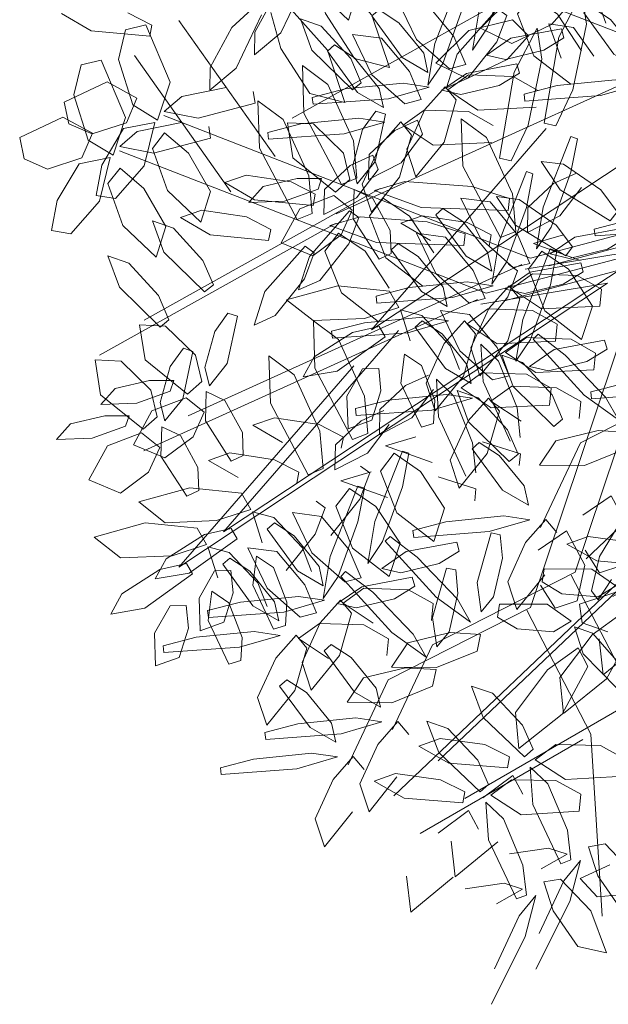
# Model space of a CAD drawing. Units: inches. Extents: x -48 to 50072, y 0 to 21068.
# Tile 72 of 75: x 2857 to 5091, y 14380 to 18117. Entities that reach past the tile are written whole.
import ezdxf

# ---------------------------------------------------------------- set-up
doc = ezdxf.new("R2010")
doc.units = ezdxf.units.IN
doc.header["$MEASUREMENT"] = 0
doc.layers.add('L-PLNT', color=94, linetype='Continuous', lineweight=13)

# ---------------------------------------------------------------- blocks, each defined once
blk = doc.blocks.new('A$C173E365C')
for p, q in [((1.5761, 3.6983), (1.6808, 3.966)), ((0.5021, 3.767), (0.4099, 3.8142)), ((0.8813, 3.8284), (0.8053, 3.758)), ((0.9917, 3.6783), (0.9528, 3.8156)), ((1.0318, 3.8259), (1.1681, 3.6723)), ((1.6811, 3.8304), (1.6056, 3.6222)), ((0.1587, 3.8117), (0.2714, 3.7462)), ((0.8218, 3.6045), (0.9181, 3.8063)), ((1.8711, 3.7875), (1.7053, 3.7467)), ((1.9311, 3.7273), (1.8711, 3.7875)), ((0.2714, 3.7462), (0.494, 3.7249)), ((0.494, 3.7249), (0.5021, 3.767)), ((0.8053, 3.758), (0.7232, 3.6071)), ((1.7053, 3.7467), (1.5796, 3.6226)), ((1.9642, 3.756), (1.8772, 3.589)), ((1.9823, 3.6377), (1.9642, 3.756)), ((2.0085, 3.7729), (2.1025, 3.7585)), ((2.0553, 3.6421), (2.0085, 3.7729)), ((2.1025, 3.7585), (2.18, 3.6496)), ((1.2636, 3.7321), (1.3739, 3.7178)), ((1.3371, 3.579), (1.2636, 3.7321)), ((1.3739, 3.7178), (1.4793, 3.5913)), ((1.8499, 3.6368), (1.9311, 3.7273)), ((1.1017, 3.5078), (0.9917, 3.6783)), ((1.168, 3.669), (1.1949, 3.6927)), ((1.2827, 3.5117), (1.168, 3.669)), ((1.1681, 3.6723), (1.2347, 3.4738)), ((1.1949, 3.6927), (1.2703, 3.6435)), ((1.5498, 3.5395), (1.5761, 3.6983)), ((0.3098, 3.635), (0.2331, 3.6169)), ((0.4015, 3.4171), (0.3098, 3.635)), ((0.8011, 3.1351), (0.4353, 3.6521)), ((1.2703, 3.6435), (1.3645, 3.5273)), ((1.6992, 3.5646), (1.8499, 3.6368)), ((1.93, 3.3883), (1.9823, 3.6377)), ((0.2331, 3.6169), (0.2056, 3.5033)), ((0.7232, 3.6071), (0.7217, 3.5211)), ((0.7217, 3.5211), (0.8218, 3.6045)), ((1.4793, 3.5913), (1.5243, 3.4847)), ((1.6056, 3.6222), (1.5498, 3.5395)), ((1.5796, 3.6226), (1.6992, 3.5646)), ((1.6957, 3.5841), (1.8871, 3.62)), ((1.8772, 3.589), (1.8217, 3.2626)), ((1.8871, 3.62), (1.8969, 3.5855)), ((1.4619, 3.4687), (1.3371, 3.579)), ((1.6023, 3.5204), (1.6957, 3.5841)), ((1.8969, 3.5855), (1.8201, 3.5387)), ((1.3645, 3.5273), (1.3805, 3.4548)), ((1.6746, 3.5036), (1.6023, 3.5204)), ((1.8201, 3.5387), (1.6746, 3.5036)), ((0.2056, 3.5033), (0.2599, 3.3313)), ((0.9042, 3.4803), (0.91, 3.3006)), ((1.0001, 3.4088), (0.9042, 3.4803)), ((1.2347, 3.4738), (1.1017, 3.5078)), ((1.3805, 3.4548), (1.2827, 3.5117)), ((1.5243, 3.4847), (1.4619, 3.4687)), ((1.535, 3.4449), (1.4557, 3.388)), ((1.704, 3.4392), (1.535, 3.4449)), ((1.7972, 3.3865), (1.704, 3.4392)), ((0.1633, 3.4186), (0, 3.3413)), ((0.2759, 3.3573), (0.1633, 3.4186)), ((0.3545, 3.2734), (0.4015, 3.4171)), ((1.0981, 3.1948), (1.0001, 3.4088)), ((1.0667, 3.3925), (1.2871, 3.414)), ((1.2871, 3.414), (1.3858, 3.3992)), ((0.6146, 3.3975), (0.4463, 3.3632)), ((0.7247, 3.338), (0.7176, 3.3828)), ((0.9414, 3.36), (1.0667, 3.3925)), ((1.3858, 3.3992), (1.2311, 3.3546)), ((1.3693, 3.3133), (1.4462, 3.3998)), ((1.4462, 3.3998), (1.4875, 3.3503)), ((1.4557, 3.388), (1.5699, 3.312)), ((1.8657, 3.2519), (1.93, 3.3883)), ((0, 3.3413), (0.0175, 3.2595)), ((0.2358, 3.2632), (0.2759, 3.3573)), ((0.2599, 3.3313), (0.3545, 3.2734)), ((0.4463, 3.3632), (0.3797, 3.3068)), ((0.5083, 3.2812), (0.7247, 3.338)), ((0.9444, 3.334), (0.9414, 3.36)), ((1.2311, 3.3546), (0.9444, 3.334)), ((1.4875, 3.3503), (1.4417, 3.1902)), ((1.7703, 2.7497), (0.3786, 3.2908)), ((0.3797, 3.3068), (0.5083, 3.2812)), ((0.91, 3.3006), (1.0531, 3.0294)), ((1.3005, 3.1637), (1.3693, 3.3133)), ((1.5699, 3.312), (1.7909, 3.3223)), ((0.0175, 3.2595), (0.1061, 3.221)), ((0.1061, 3.221), (0.2358, 3.2632)), ((0.3439, 3.2644), (0.2256, 3.2413)), ((0.3033, 3.0996), (0.3439, 3.2644)), ((1.2545, 3.2344), (1.341, 3.2734)), ((1.341, 3.2734), (1.3605, 3.2197)), ((1.8217, 3.2626), (1.8657, 3.2519)), ((0.2256, 3.2413), (0.1424, 3.102)), ((0.381, 3.2251), (0.3349, 3.1664)), ((0.4716, 3.1476), (0.381, 3.2251)), ((1.1569, 3.1431), (1.2545, 3.2344)), ((1.3605, 3.2197), (1.2785, 3.1117)), ((1.1106, 3.0527), (1.0981, 3.1948)), ((1.4417, 3.1902), (1.335, 3.058)), ((1.8185, 2.9435), (1.9233, 3.2112)), ((1.9233, 3.2112), (1.9481, 3.2027)), ((1.9481, 3.2027), (1.9235, 3.0756)), ((0.3349, 3.1664), (0.3919, 3.0064)), ((0.5547, 3.0026), (0.4716, 3.1476)), ((1.1551, 3.048), (1.1569, 3.1431)), ((1.335, 3.058), (1.3005, 3.1637)), ((1.2785, 3.1117), (1.1551, 3.048)), ((1.81, 3.1168), (1.8824, 3.0084)), ((1.8955, 3.1061), (1.81, 3.1168)), ((2.0367, 3.0085), (1.8955, 3.1061)), ((0.1424, 3.102), (0.1209, 2.9878)), ((0.1943, 2.9757), (0.3033, 3.0996)), ((0.6912, 3.0649), (0.6098, 3.0369)), ((0.861, 3.0394), (0.6912, 3.0649)), ((1.9235, 3.0756), (1.8481, 2.8674)), ((0.6098, 3.0369), (0.7225, 2.9714)), ((0.9531, 2.9922), (0.861, 3.0394)), ((1.0531, 3.0294), (1.1106, 3.0527)), ((1.2926, 3.04), (1.1777, 3.0063)), ((1.5467, 3.0213), (1.2926, 3.04)), ((2.865, 3.0377), (1.7703, 2.7497)), ((1.1988, 3.0143), (0.3031, 2.5146)), ((0.3919, 3.0064), (0.518, 2.8861)), ((0.518, 2.8861), (0.5547, 3.0026)), ((0.945, 2.95), (0.9531, 2.9922)), ((1.1777, 3.0063), (1.3548, 2.9424)), ((1.6904, 2.9757), (1.5467, 3.0213)), ((1.8398, 2.7206), (2.867, 2.9966)), ((1.8824, 3.0084), (2.0729, 2.8913)), ((2.0987, 2.9256), (2.0367, 3.0085)), ((2.1813, 2.9933), (2.3067, 3.0258)), ((2.1844, 2.9673), (2.1813, 2.9933)), ((0.1209, 2.9878), (0.1943, 2.9757)), ((0.7225, 2.9714), (0.945, 2.95)), ((1.2105, 2.9773), (1.1589, 2.9099)), ((1.311, 2.9089), (1.2105, 2.9773)), ((1.5061, 2.9774), (1.6163, 2.963)), ((1.5795, 2.8242), (1.5061, 2.9774)), ((1.6163, 2.963), (1.7218, 2.8365)), ((1.6857, 2.9306), (1.6904, 2.9757)), ((2.471, 2.9879), (2.1844, 2.9673)), ((0.9304, 2.7565), (1.0834, 2.929)), ((1.0834, 2.929), (1.118, 2.9036)), ((1.3548, 2.9424), (1.6857, 2.9306)), ((1.4104, 2.9143), (1.4373, 2.9379)), ((1.4373, 2.9379), (1.5127, 2.8887)), ((1.7923, 2.7847), (1.8185, 2.9435)), ((2.0729, 2.8913), (2.0987, 2.9256)), ((0.335, 2.8916), (0.3785, 2.7727)), ((0.4142, 2.8638), (0.335, 2.8916)), ((1.118, 2.9036), (1.0805, 2.8038)), ((1.1589, 2.9099), (1.2213, 2.751)), ((1.4026, 2.7692), (1.311, 2.9089)), ((1.5252, 2.7569), (1.4104, 2.9143)), ((1.5127, 2.8887), (1.6069, 2.7725)), ((0.5263, 2.7411), (0.4142, 2.8638)), ((1.8481, 2.8674), (1.7923, 2.7847)), ((1.9381, 2.8293), (2.1295, 2.8652)), ((2.1295, 2.8652), (2.1393, 2.8307)), ((1.0805, 2.8038), (0.97, 2.6654)), ((1.7044, 2.7139), (1.5795, 2.8242)), ((1.7218, 2.8365), (1.7668, 2.7299)), ((1.8447, 2.7656), (1.9381, 2.8293)), ((2.1393, 2.8307), (2.0625, 2.7839)), ((0.3785, 2.7727), (0.533, 2.6213)), ((0.6043, 1.7104), (2.2312, 2.7878)), ((1.6069, 2.7725), (1.6229, 2.7)), ((1.7499, 2.7082), (2.2312, 2.7878)), ((2.0625, 2.7839), (1.917, 2.7488)), ((2.3552, 2.7991), (1.9394, 1.5574)), ((0.566, 2.6488), (0.5263, 2.7411)), ((0.8898, 2.6288), (0.9304, 2.7565)), ((1.2213, 2.751), (1.361, 2.6428)), ((1.6229, 2.7), (1.5252, 2.7569)), ((1.7668, 2.7299), (1.7044, 2.7139)), ((1.917, 2.7488), (1.8447, 2.7656)), ((1.7373, 2.7261), (0.4708, 2.1514)), ((0.97, 2.6654), (0.8898, 2.6288)), ((1.3092, 2.6377), (1.5295, 2.6592)), ((1.5295, 2.6592), (1.6282, 2.6444)), ((1.7774, 2.6902), (1.6981, 2.6332)), ((1.9465, 2.6844), (1.7774, 2.6902)), ((2.0396, 2.6317), (1.9465, 2.6844)), ((0.533, 2.6213), (0.566, 2.6488)), ((1.1838, 2.6052), (1.3092, 2.6377)), ((1.6282, 2.6444), (1.4735, 2.5998)), ((1.6117, 2.5585), (1.6886, 2.645)), ((1.6886, 2.645), (1.7299, 2.5955)), ((1.6981, 2.6332), (1.8123, 2.5572)), ((2.0333, 2.5676), (2.0396, 2.6317)), ((1.1868, 2.5792), (1.1838, 2.6052)), ((1.4735, 2.5998), (1.1868, 2.5792)), ((1.7299, 2.5955), (1.6841, 2.4354)), ((1.543, 2.4089), (1.6117, 2.5585)), ((1.8123, 2.5572), (2.0333, 2.5676)), ((0.6212, 2.541), (0.5713, 2.4712)), ((0.6187, 2.3492), (0.6575, 2.5291)), ((0.6575, 2.5291), (0.6212, 2.541)), ((0.9457, 2.5118), (0.9515, 2.3321)), ((1.0416, 2.4403), (0.9457, 2.5118)), ((0.2859, 2.4963), (0.3067, 2.3639)), ((0.385, 2.492), (0.2859, 2.4963)), ((0.4982, 2.3815), (0.385, 2.492)), ((0.5713, 2.4712), (0.5336, 2.335)), ((1.2683, 2.4746), (0.6043, 1.7104)), ((1.1396, 2.2263), (1.0416, 2.4403)), ((1.6841, 2.4354), (1.5774, 2.3032)), ((1.7548, 2.448), (1.6755, 2.391)), ((1.9238, 2.4422), (1.7548, 2.448)), ((2.017, 2.3895), (1.9238, 2.4422)), ((1.5774, 2.3032), (1.543, 2.4089)), ((1.5819, 2.4233), (1.5903, 2.2808)), ((1.6482, 2.3591), (1.5819, 2.4233)), ((2.168, 2.3752), (2.2934, 2.4077)), ((0.3067, 2.3639), (0.4685, 2.2336)), ((0.5224, 2.281), (0.4982, 2.3815)), ((1.7194, 2.1819), (1.6482, 2.3591)), ((1.6606, 2.381), (1.7041, 2.2621)), ((1.7398, 2.3532), (1.6606, 2.381)), ((1.6755, 2.391), (1.7896, 2.315)), ((2.0106, 2.3253), (2.017, 2.3895)), ((2.1711, 2.3492), (2.168, 2.3752)), ((2.4578, 2.3698), (2.1711, 2.3492)), ((0.5336, 2.335), (0.5509, 2.2648)), ((0.5509, 2.2648), (0.6187, 2.3492)), ((0.9515, 2.3321), (1.0945, 2.0609)), ((1.8519, 2.2306), (1.7398, 2.3532)), ((1.7896, 2.315), (2.0106, 2.3253)), ((0.1931, 2.2544), (0.3233, 2.2846)), ((0.3233, 2.2846), (0.4155, 2.2847)), ((0.4155, 2.2847), (0.4018, 2.2445)), ((0.4685, 2.2336), (0.5224, 2.281)), ((1.296, 2.2658), (1.3825, 2.3049)), ((1.5903, 2.2808), (1.6932, 2.0548)), ((0.1391, 2.1939), (0.1931, 2.2544)), ((0.4018, 2.2445), (0.2751, 2.199)), ((0.5393, 2.2429), (0.5357, 2.1317)), ((0.6102, 2.2095), (0.5393, 2.2429)), ((1.1984, 2.1746), (1.296, 2.2658)), ((1.402, 2.2512), (1.32, 2.1432)), ((1.7041, 2.2621), (1.8586, 2.1107)), ((0.4623, 2.22), (0.3328, 2.17)), ((0.5315, 2.1646), (0.4623, 2.22)), ((0.6762, 2.0877), (0.6102, 2.2095)), ((1.1521, 2.0842), (1.1396, 2.2263)), ((1.8916, 2.1383), (1.8519, 2.2306)), ((0.2751, 2.199), (0.1391, 2.1939)), ((0.3328, 2.17), (0.2624, 2.0408)), ((1.1966, 2.0795), (1.1984, 2.1746)), ((2.8463, 2.1989), (1.4196, 0.8417)), ((1.7313, 2.0686), (1.7194, 2.1819)), ((0.4892, 2.071), (0.5315, 2.1646)), ((0.5357, 2.1317), (0.634, 1.9795)), ((0.7977, 2.1434), (0.7163, 2.1154)), ((0.9675, 2.1179), (0.7977, 2.1434)), ((1.32, 2.1432), (1.1966, 2.0795)), ((1.8586, 2.1107), (1.8916, 2.1383)), ((0.7163, 2.1154), (0.829, 2.0499)), ((1.0597, 2.0707), (0.9675, 2.1179)), ((0.3821, 1.9912), (0.4892, 2.071)), ((0.6795, 2.0007), (0.6762, 2.0877)), ((1.0515, 2.0285), (1.0597, 2.0707)), ((1.0945, 2.0609), (1.1521, 2.0842)), ((1.3341, 2.0715), (1.2192, 2.0378)), ((0.2624, 2.0408), (0.3821, 1.9912)), ((1.2192, 2.0378), (1.3963, 1.9738)), ((1.7319, 2.0072), (1.5882, 2.0527)), ((0.634, 1.9795), (0.6795, 2.0007)), ((1.1788, 1.75), (1.2835, 2.0176)), ((1.252, 2.0088), (1.2003, 1.9413)), ((1.3525, 1.9404), (1.252, 2.0088)), ((1.2835, 2.0176), (1.3084, 2.0092)), ((1.3084, 2.0092), (1.2838, 1.882)), ((1.7272, 1.9621), (1.7319, 2.0072)), ((1.1249, 1.9605), (1.1595, 1.9351)), ((1.1595, 1.9351), (1.122, 1.8353)), ((1.2003, 1.9413), (1.2628, 1.7825)), ((1.4441, 1.8006), (1.3525, 1.9404)), ((0.4765, 1.8776), (0.2828, 1.8241)), ((0.6731, 1.8578), (0.4765, 1.8776)), ((1.2838, 1.882), (1.2083, 1.6739)), ((0.7086, 1.7956), (0.6731, 1.8578)), ((1.122, 1.8353), (1.0115, 1.6969)), ((2.0757, 1.8477), (1.9687, 1.7746)), ((2.1454, 1.7181), (2.0757, 1.8477)), ((2.2012, 1.7506), (2.2713, 1.8672)), ((0.2828, 1.8241), (0.3831, 1.7455)), ((0.5786, 1.7535), (0.7086, 1.7956)), ((1.4025, 1.6743), (1.4441, 1.8006)), ((0.7146, 1.7865), (0.7517, 1.6694)), ((0.7954, 1.7653), (0.7146, 1.7865)), ((0.9039, 1.6505), (0.7954, 1.7653)), ((0.8663, 1.7838), (0.9766, 1.7694)), ((0.9398, 1.6306), (0.8663, 1.7838)), ((0.9766, 1.7694), (1.082, 1.643)), ((1.2628, 1.7825), (1.4025, 1.6743)), ((0.3831, 1.7455), (0.5786, 1.7535)), ((0.6336, 1.7239), (0.5323, 1.7006)), ((0.6563, 1.6847), (0.6336, 1.7239)), ((0.7707, 1.7207), (0.7976, 1.7444)), ((0.8854, 1.5633), (0.7707, 1.7207)), ((0.7976, 1.7444), (0.873, 1.6952)), ((1.1525, 1.5912), (1.1788, 1.75)), ((2.1701, 1.6197), (2.2012, 1.7506)), ((0.5323, 1.7006), (0.3875, 1.6083)), ((0.4748, 1.554), (0.6563, 1.6847)), ((0.873, 1.6952), (0.9672, 1.5789)), ((1.2186, 1.6751), (1.2372, 1.6936)), ((1.2372, 1.6936), (1.3402, 1.6151)), ((1.5673, 1.5189), (1.6202, 1.7064)), ((1.6202, 1.7064), (1.6554, 1.6999)), ((1.6554, 1.6999), (1.6633, 1.6102)), ((2.1165, 1.5824), (2.1454, 1.7181)), ((0.9389, 1.5601), (0.9039, 1.6505)), ((1.2083, 1.6739), (1.1525, 1.5912)), ((1.412, 1.4625), (1.2186, 1.6751)), ((1.2984, 1.6358), (1.4898, 1.6716)), ((1.4898, 1.6716), (1.4996, 1.6372)), ((2.2466, 1.6635), (2.1962, 1.5862)), ((0.3875, 1.6083), (0.3455, 1.5318)), ((0.7299, 1.6188), (0.7156, 1.5079)), ((0.7942, 1.5751), (0.7299, 1.6188)), ((1.0646, 1.5204), (0.9398, 1.6306)), ((1.082, 1.643), (1.127, 1.5364)), ((1.205, 1.572), (1.2984, 1.6358)), ((1.3402, 1.6151), (1.4933, 1.4552)), ((1.4996, 1.6372), (1.4228, 1.5903)), ((1.6633, 1.6102), (1.6301, 1.4643)), ((1.977, 1.6413), (2.0322, 1.5547)), ((2.322, 1.634), (2.1245, 1.5697)), ((2.1962, 1.5862), (2.1701, 1.6197)), ((0.8451, 1.4434), (0.7942, 1.5751)), ((0.9672, 1.5789), (0.9832, 1.5064)), ((1.2773, 1.5553), (1.205, 1.572)), ((1.4228, 1.5903), (1.2773, 1.5553)), ((1.8212, 1.57), (1.8141, 1.5204)), ((2.0024, 1.5691), (1.8212, 1.57)), ((2.0322, 1.5547), (2.1165, 1.5824)), ((0.3455, 1.5318), (0.4748, 1.554)), ((0.5709, 1.5628), (0.5116, 1.4589)), ((0.6323, 1.564), (0.5709, 1.5628)), ((0.6407, 1.4789), (0.6323, 1.564)), ((0.9832, 1.5064), (0.8854, 1.5633)), ((1.127, 1.5364), (1.0646, 1.5204)), ((1.9394, 1.5574), (1.3983, 1.2817)), ((1.9246, 1.5469), (2.168, 1.0766)), ((2.0936, 1.5054), (2.0024, 1.5691)), ((2.1245, 1.5697), (2.1347, 1.4988)), ((0.7156, 1.5079), (0.7942, 1.3411)), ((1.1377, 1.4966), (1.0584, 1.4396)), ((1.3067, 1.4909), (1.1377, 1.4966)), ((1.583, 1.4069), (1.5673, 1.5189)), ((1.8141, 1.5204), (1.8887, 1.4756)), ((2.0269, 1.4643), (2.0936, 1.5054)), ((2.1347, 1.4988), (2.232, 1.464)), ((0.5116, 1.4589), (0.5161, 1.3349)), ((0.6055, 1.3674), (0.6407, 1.4789)), ((0.6694, 1.4442), (0.8898, 1.4657)), ((0.8898, 1.4657), (0.9885, 1.4509)), ((1.3999, 1.4382), (1.3067, 1.4909)), ((1.5426, 1.3685), (1.412, 1.4625)), ((1.6301, 1.4643), (1.583, 1.4069)), ((1.8887, 1.4756), (2.0269, 1.4643)), ((2.1056, 1.4837), (2.1392, 1.3808)), ((2.1738, 1.4598), (2.1056, 1.4837)), ((2.2672, 1.3538), (2.1738, 1.4598)), ((0.5441, 1.4117), (0.6694, 1.4442)), ((0.9885, 1.4509), (0.8338, 1.4063)), ((0.8397, 1.3557), (0.8451, 1.4434)), ((0.972, 1.3649), (1.0489, 1.4514)), ((1.0489, 1.4514), (1.0902, 1.402)), ((1.0584, 1.4396), (1.1726, 1.3636)), ((1.3936, 1.374), (1.3999, 1.4382)), ((1.4933, 1.4552), (1.5426, 1.3685)), ((0.5471, 1.3856), (0.5441, 1.4117)), ((0.8338, 1.4063), (0.5471, 1.3856)), ((1.0902, 1.402), (1.0444, 1.2418)), ((2.0041, 1.3199), (2.1197, 1.4035)), ((2.1197, 1.4035), (2.1565, 1.3328)), ((0.5161, 1.3349), (0.6055, 1.3674)), ((0.7942, 1.3411), (0.8397, 1.3557)), ((0.9032, 1.2153), (0.972, 1.3649)), ((2.1392, 1.3808), (2.2686, 1.2499)), ((1.3047, 1.2899), (1.4649, 1.3283)), ((1.4649, 1.3283), (1.5804, 1.3213)), ((1.5804, 1.3213), (1.567, 1.2582)), ((1.8815, 1.1582), (2.0041, 1.3199)), ((2.1565, 1.3328), (2.0589, 1.1522)), ((0.9868, 1.2587), (1.0136, 1.2825)), ((1.0136, 1.2825), (1.0892, 1.2337)), ((1.2429, 1.1975), (1.3047, 1.2899)), ((1.3983, 1.2817), (1.2465, 0.9602)), ((1.0444, 1.2418), (0.9377, 1.1096)), ((1.1023, 1.1019), (0.9868, 1.2587)), ((1.0892, 1.2337), (1.184, 1.1179)), ((1.567, 1.2582), (1.4128, 1.1953)), ((0.9377, 1.1096), (0.9032, 1.2153)), ((1.4128, 1.1953), (1.2429, 1.1975)), ((1.5457, 1.1248), (1.5908, 1.0066)), ((1.6253, 1.0981), (1.5457, 1.1248)), ((1.8952, 1.0216), (1.8815, 1.1582)), ((2.0589, 1.1522), (1.8952, 1.0216)), ((1.2004, 1.0455), (1.1023, 1.1019)), ((1.184, 1.1179), (1.2004, 1.0455)), ((1.7391, 0.9771), (1.6253, 1.0981)), ((2.1382, 1.0556), (1.5206, 0.6989)), ((2.168, 1.0766), (2.2114, 0.3846)), ((0.7618, 0.9485), (0.887, 0.9816)), ((0.887, 0.9816), (1.1072, 1.0043)), ((1.206, 0.99), (1.0515, 0.9446)), ((1.1072, 1.0043), (1.206, 0.99)), ((1.19, 0.904), (1.2664, 0.9909)), ((1.2664, 0.9909), (1.308, 0.9417)), ((1.5908, 1.0066), (1.7474, 0.8573)), ((1.78, 0.8853), (1.7391, 0.9771)), ((0.765, 0.9225), (0.7618, 0.9485)), ((1.0515, 0.9446), (0.765, 0.9225)), ((1.122, 0.754), (1.19, 0.904)), ((1.427, 0.9262), (1.346, 0.8971)), ((1.346, 0.8971), (1.4596, 0.8332)), ((1.5971, 0.9031), (1.427, 0.9262)), ((1.6899, 0.8572), (1.5971, 0.9031)), ((1.8666, 0.9029), (1.7881, 0.8449)), ((2.0357, 0.8995), (1.8666, 0.9029)), ((2.1296, 0.8481), (2.0357, 0.8995)), ((1.7474, 0.8573), (1.78, 0.8853)), ((1.4596, 0.8332), (1.6824, 0.8149)), ((1.6824, 0.8149), (1.6899, 0.8572)), ((1.7881, 0.8449), (1.9033, 0.7704)), ((2.1241, 0.7839), (2.1296, 0.8481)), ((1.5889, 0.7006), (1.7034, 0.7857)), ((1.7034, 0.7857), (1.7411, 0.7156)), ((1.7691, 0.8178), (1.7794, 0.6754)), ((1.8363, 0.7544), (1.7691, 0.8178)), ((1.157, 0.6485), (1.122, 0.754)), ((1.263, 0.7812), (1.157, 0.6485)), ((1.9099, 0.5783), (1.8363, 0.7544)), ((1.9033, 0.7704), (2.1241, 0.7839)), ((1.7794, 0.6754), (1.8855, 0.4509)), ((1.9234, 0.4652), (1.9099, 0.5783)), ((2.2401, 0.5805), (2.1275, 0.5283)), ((1.4842, 0.4008), (1.4686, 0.5372)), ((1.646, 0.5336), (1.4842, 0.4008)), ((1.9898, 0.5157), (2.0534, 0.526)), ((2.0534, 0.526), (2.1678, 0.4049)), ((2.1275, 0.5283), (2.1921, 0.4585)), ((1.6904, 0.4887), (1.8385, 0.5105)), ((1.909, 0.4873), (1.8102, 0.4322)), ((1.8385, 0.5105), (1.909, 0.4873)), ((2.025, 0.4055), (1.9898, 0.5157)), ((1.8855, 0.4509), (1.9234, 0.4652)), ((1.8964, 0.3862), (1.9595, 0.4635)), ((1.9595, 0.4635), (1.9189, 0.3077)), ((2.1921, 0.4585), (2.3085, 0.4692)), ((1.8025, 0.1857), (1.8964, 0.3862)), ((2.1186, 0.27), (2.025, 0.4055)), ((2.1678, 0.4049), (2.2271, 0.2457)), ((1.9189, 0.3077), (1.7905, 0.0506)), ((2.2271, 0.2457), (2.1186, 0.27))]:
    blk.add_line(p, q)

msp = doc.modelspace()

# ---------------------------------------------------------------- block references
at = {"layer": 'L-PLNT', "xscale": 1000, "yscale": 1000, "zscale": 1000}
for p in [(3587.393, 15229.446), (3025.86, 14462.551), (2856.783, 14329.296)]:
    msp.add_blockref('A$C173E365C', p, dxfattribs=at)

doc.saveas('drawing.dxf')
